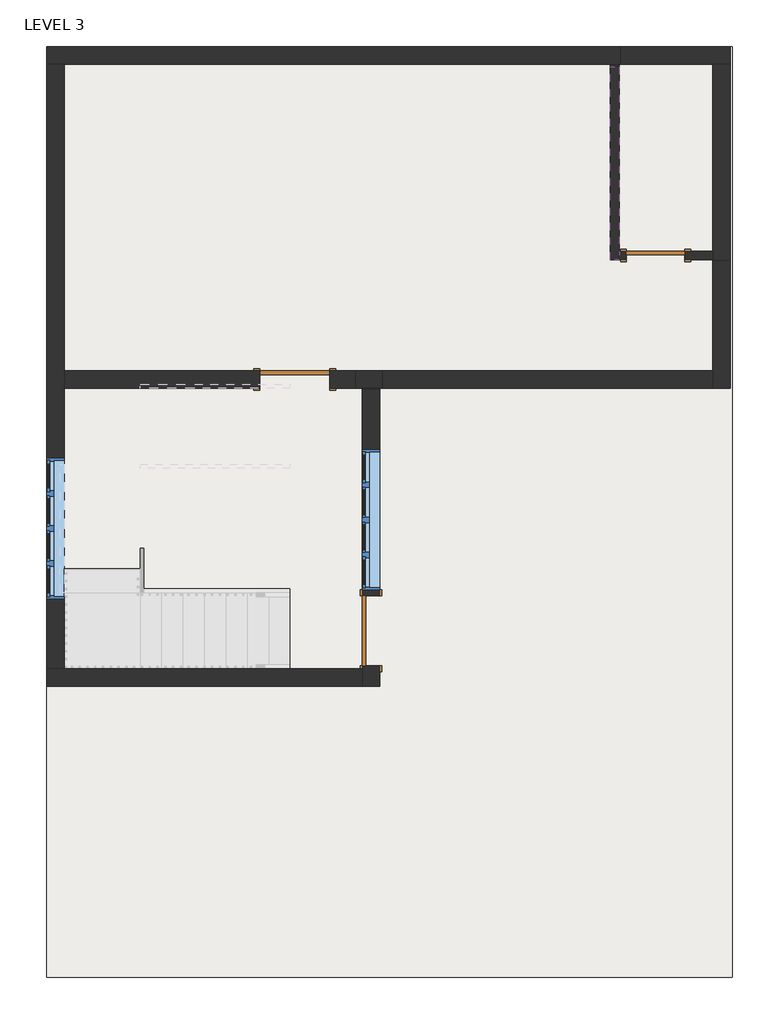
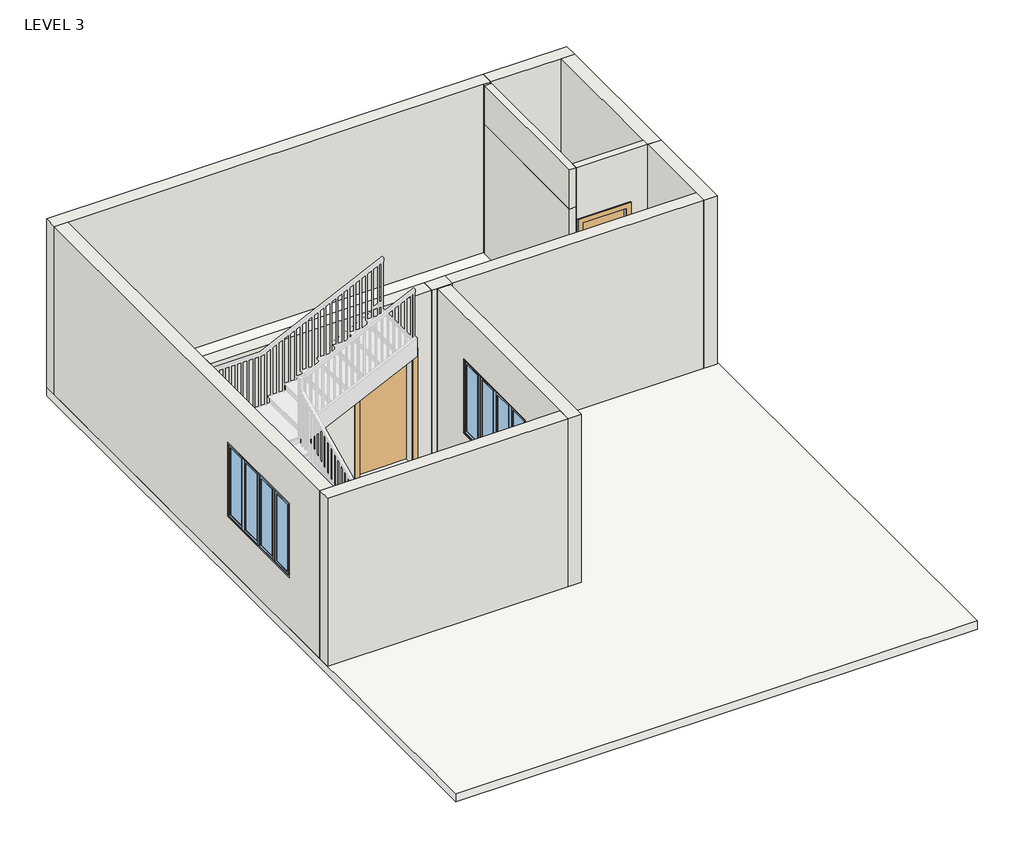
# One storey, part 1 of 3: 15 walls, 3 doors, 2 windows, 1 slab.
"""IFC4 building model written with IfcOpenShell, lengths in millimetres."""

from ifc_helpers import new_model, si_unit, frame, origin, place, context, project, spatial, polyline, outline, extrude, faceted_brep, transform, mapped, element, save
from components import door_feaa5179, door_f2b275c1, single_flush_door_3_89fc3733, window_5487fb6d

model = new_model("IFC4")

# Units and contexts
model_context = context("Model", 3, world=origin())
ifc_project = project(units=[si_unit("LENGTHUNIT", "METRE", prefix="MILLI")], contexts=[model_context])

# Site, building, storey
site = spatial("IfcSite", under=ifc_project)
building = spatial("IfcBuilding", under=site)
storey = spatial("IfcBuildingStorey", under=building, Name="LEVEL 3", Elevation=6248.4)

# Doors
placement = place(None, origin())
door_shape = door_feaa5179(model_context)
element("IfcDoor", 1, ObjectType="Door-Single-Flush_Panel_Double-Acting : 36\" x 80\"", at=placement, inside=storey, context=model_context, shape_type="MappedRepresentation", body=[
    mapped(door_shape, transform((-18715.7789184, -623.1399287, 6248.4), x_axis=(0.0, 1.0, 0.0), y_axis=(-1.0, 0.0, 0.0), z_axis=(0.0, 0.0, 1.0))),
])
door_2_shape = door_f2b275c1(model_context)
element("IfcDoor", 2, ObjectType="Single-Flush : door 2'6\"", at=placement, inside=storey, context=model_context, shape_type="MappedRepresentation", body=[
    mapped(door_2_shape, transform((-15001.0289184, 4272.7100713, 6248.4), x_axis=(-1.0, 0.0, 0.0), y_axis=(0.0, -1.0, 0.0), z_axis=(0.0, 0.0, 1.0))),
])
single_flush_door_3_shape = single_flush_door_3_89fc3733(model_context)
element("IfcDoor", 3, ObjectType="Single-Flush : door 3'", at=placement, inside=storey, context=model_context, shape_type="MappedRepresentation", body=[
    mapped(single_flush_door_3_shape, transform((-19706.3789184, 2653.4600713, 6248.4), x_axis=(1.0, 0.0, 0.0), y_axis=(0.0, 1.0, 0.0), z_axis=(0.0, 0.0, 1.0))),
])

# Slab
element("IfcSlab", 4, ObjectType="floor 6\"", at=placement, inside=storey, context=model_context, shape_type="SweptSolid", body=[
    extrude(outline(polyline([(-14004.0789184, 6996.8600713), (-14004.0789184, -5144.3399287), (-22944.8789184, -5144.3399287), (-22944.8789184, 6996.8600713), (-14004.0789184, 6996.8600713)])), frame((0.0, 0.0, 6096.0), z_axis=(0.0, 0.0, 1.0), x_axis=(1.0, 0.0, 0.0)), (0.0, 0.0, 1.0), 152.4),
])

# Walls
element("IfcWall", 5, ObjectType="WALL 4.5\"", at=placement, inside=storey, context=model_context, shape_type="Brep", body=[
    faceted_brep([(-15591.5789184, 6768.2600713, 6248.4), (-15591.5789184, 6730.1600713, 6248.4), (-15591.5789184, 6730.1600713, 8585.2), (-15591.5789184, 6730.1600713, 9296.4), (-15591.5789184, 6768.2600713, 9296.4), (-15477.2789184, 6768.2600713, 6248.4), (-15477.2789184, 6768.2600713, 9296.4), (-15477.2789184, 6730.1600713, 9296.4), (-15477.2789184, 6730.1600713, 8585.2), (-15477.2789184, 6730.1600713, 6248.4)], [[[0, 1, 2, 3, 4]], [[5, 6, 7, 8, 9]], [[1, 0, 5, 9]], [[4, 3, 7, 6]], [[0, 4, 6, 5]], [[1, 9, 8, 7, 3, 2]]]),
])
element("IfcWall", 6, ObjectType="WALL 4.5\"", at=placement, inside=storey, context=model_context, shape_type="Brep", body=[
    faceted_brep([(-14258.0789184, 4215.5600713, 9296.4), (-15477.2789184, 4215.5600713, 9296.4), (-15477.2789184, 4215.5600713, 8585.2), (-15477.2789184, 4215.5600713, 6248.4), (-15382.0289184, 4215.5600713, 6248.4), (-15382.0289184, 4215.5600713, 8280.4), (-14620.0289184, 4215.5600713, 8280.4), (-14620.0289184, 4215.5600713, 6248.4), (-14258.0789184, 4215.5600713, 6248.4), (-15477.2789184, 4329.8600713, 9296.4), (-14258.0789184, 4329.8600713, 9296.4), (-14258.0789184, 4329.8600713, 6248.4), (-14620.0289184, 4329.8600713, 6248.4), (-14620.0289184, 4329.8600713, 8280.4), (-15382.0289184, 4329.8600713, 8280.4), (-15382.0289184, 4329.8600713, 6248.4), (-15477.2789184, 4329.8600713, 6248.4)], [[[0, 1, 2, 3, 4, 5, 6, 7, 8]], [[9, 10, 11, 12, 13, 14, 15, 16]], [[3, 16, 15, 4]], [[11, 8, 7, 12]], [[1, 0, 10, 9]], [[0, 8, 11, 10]], [[14, 5, 4, 15]], [[6, 13, 12, 7]], [[13, 6, 5, 14]], [[1, 9, 16, 3, 2]]]),
])
element("IfcWall", 7, ObjectType="WALL 4.5\"", at=placement, inside=storey, context=model_context, shape_type="Brep", body=[
    faceted_brep([(-15591.5789184, 6730.1600713, 6248.4), (-15591.5789184, 4215.5600713, 6248.4), (-15591.5789184, 4215.5600713, 8585.2), (-15591.5789184, 6730.1600713, 8585.2), (-15477.2789184, 6730.1600713, 6248.4), (-15477.2789184, 6730.1600713, 8585.2), (-15477.2789184, 4215.5600713, 8585.2), (-15477.2789184, 4215.5600713, 6248.4), (-15477.2789184, 4329.8600713, 6248.4)], [[[0, 1, 2, 3]], [[4, 5, 6, 7, 8]], [[1, 0, 4, 8, 7]], [[3, 2, 6, 5]], [[0, 3, 5, 4]], [[2, 1, 7, 6]]]),
])
element("IfcWall", 8, ObjectType="WALL 4.5\"", at=placement, inside=storey, context=model_context, shape_type="Brep", body=[
    faceted_brep([(-15591.5789184, 6730.1600713, 8585.2), (-15591.5789184, 4215.5600713, 8585.2), (-15591.5789184, 4215.5600713, 9296.4), (-15591.5789184, 6730.1600713, 9296.4), (-15477.2789184, 6730.1600713, 8585.2), (-15477.2789184, 6730.1600713, 9296.4), (-15477.2789184, 4329.8600713, 9296.4), (-15477.2789184, 4215.5600713, 9296.4), (-15477.2789184, 4215.5600713, 8585.2)], [[[0, 1, 2, 3]], [[4, 5, 6, 7, 8]], [[1, 0, 4, 8]], [[3, 2, 7, 6, 5]], [[0, 3, 5, 4]], [[2, 1, 8, 7]]]),
])
element("IfcWall", 9, ObjectType="WALL 9\"", at=placement, inside=storey, context=model_context, shape_type="Brep", body=[
    faceted_brep([(-22944.8789184, 6768.2600713, 6248.4), (-22716.2789184, 6768.2600713, 6248.4), (-15591.5789184, 6768.2600713, 6248.4), (-15477.2789184, 6768.2600713, 6248.4), (-15464.5789184, 6768.2600713, 6248.4), (-15464.5789184, 6768.2600713, 9296.4), (-15477.2789184, 6768.2600713, 9296.4), (-15591.5789184, 6768.2600713, 9296.4), (-22716.2789184, 6768.2600713, 9296.4), (-22944.8789184, 6768.2600713, 9296.4), (-22944.8789184, 6996.8600713, 6248.4), (-22944.8789184, 6996.8600713, 9296.4), (-15464.5789184, 6996.8600713, 9296.4), (-15464.5789184, 6996.8600713, 6248.4)], [[[0, 1, 2, 3, 4, 5, 6, 7, 8, 9]], [[10, 11, 12, 13]], [[4, 3, 2, 1, 0, 10, 13]], [[5, 4, 13, 12]], [[0, 9, 11, 10]], [[9, 8, 7, 6, 5, 12, 11]]]),
])
element("IfcWall", 10, ObjectType="WALL 9\"", at=placement, inside=storey, context=model_context, shape_type="Brep", body=[
    faceted_brep([(-14258.0789184, 6768.2600713, 6248.4), (-14258.0789184, 4329.8600713, 6248.4), (-14258.0789184, 4215.5600713, 6248.4), (-14258.0789184, 4202.8600713, 6248.4), (-14258.0789184, 4202.8600713, 9296.4), (-14258.0789184, 4215.5600713, 9296.4), (-14258.0789184, 4329.8600713, 9296.4), (-14258.0789184, 6768.2600713, 9296.4), (-14029.4789184, 6768.2600713, 6248.4), (-14029.4789184, 6768.2600713, 9296.4), (-14029.4789184, 4202.8600713, 9296.4), (-14029.4789184, 4202.8600713, 6248.4)], [[[0, 1, 2, 3, 4, 5, 6, 7]], [[8, 9, 10, 11]], [[3, 2, 1, 0, 8, 11]], [[4, 3, 11, 10]], [[0, 7, 9, 8]], [[7, 6, 5, 4, 10, 9]]]),
])
element("IfcWall", 11, ObjectType="WALL 9\"", at=placement, inside=storey, context=model_context, shape_type="SweptSolid", body=[
    extrude(outline(polyline([(-18563.3789184, 2767.7600713), (-14258.0789184, 2767.7600713), (-14258.0789184, 2539.1600713), (-18563.3789184, 2539.1600713), (-18563.3789184, 2767.7600713)])), frame((0.0, 0.0, 6248.4), z_axis=(0.0, 0.0, 1.0), x_axis=(1.0, 0.0, 0.0)), (0.0, 0.0, 1.0), 3048.0),
])
element("IfcWall", 12, ObjectType="WALL 9\"", at=placement, inside=storey, context=model_context, shape_type="SweptSolid", body=[
    extrude(outline(polyline([(-18830.0789184, 2526.4600713), (-18830.0789184, 2539.1600713), (-18601.4789184, 2539.1600713), (-18601.4789184, 2526.4600713), (-18830.0789184, 2526.4600713)])), frame((0.0, 0.0, 6248.4), z_axis=(0.0, 0.0, 1.0), x_axis=(1.0, 0.0, 0.0)), (0.0, 0.0, 1.0), 3048.0),
])
element("IfcWall", 13, ObjectType="WALL 9\"", at=placement, inside=storey, context=model_context, shape_type="Brep", body=[
    faceted_brep([(-18830.0789184, -1118.4399287, 6248.4), (-22716.2789184, -1118.4399287, 6248.4), (-22944.8789184, -1118.4399287, 6248.4), (-22944.8789184, -1118.4399287, 9296.4), (-22716.2789184, -1118.4399287, 9296.4), (-19769.8789184, -1118.4399287, 9296.4), (-18830.0789184, -1118.4399287, 9296.4), (-18830.0789184, -1347.0399287, 6248.4), (-18830.0789184, -1347.0399287, 9296.4), (-22944.8789184, -1347.0399287, 9296.4), (-22944.8789184, -1347.0399287, 6248.4)], [[[0, 1, 2, 3, 4, 5, 6]], [[7, 8, 9, 10]], [[2, 1, 0, 7, 10]], [[0, 6, 8, 7]], [[3, 2, 10, 9]], [[6, 5, 4, 3, 9, 8]]]),
])
element("IfcWall", 14, ObjectType="WALL 9\"", at=placement, inside=storey, context=model_context, shape_type="Brep", body=[
    faceted_brep([(-22716.2789184, -1118.4399287, 6248.4), (-22716.2789184, 2539.1600713, 6248.4), (-22716.2789184, 2767.7600713, 6248.4), (-22716.2789184, 6768.2600713, 6248.4), (-22716.2789184, 6768.2600713, 9296.4), (-22716.2789184, 2767.7600713, 9296.4), (-22716.2789184, 2539.1600713, 9296.4), (-22716.2789184, -1118.4399287, 9296.4), (-22716.2789184, 1624.7600713, 8509.0), (-22716.2789184, 1624.7600713, 7162.8), (-22716.2789184, -204.0399287, 7162.8), (-22716.2789184, -204.0399287, 8509.0), (-22944.8789184, -1118.4399287, 6248.4), (-22944.8789184, -1118.4399287, 9296.4), (-22944.8789184, 6768.2600713, 9296.4), (-22944.8789184, 6768.2600713, 6248.4), (-22944.8789184, 1624.7600713, 8509.0), (-22944.8789184, -204.0399287, 8509.0), (-22944.8789184, -204.0399287, 7162.8), (-22944.8789184, 1624.7600713, 7162.8)], [[[0, 1, 2, 3, 4, 5, 6, 7], [8, 9, 10, 11]], [[12, 13, 14, 15], [16, 17, 18, 19]], [[3, 2, 1, 0, 12, 15]], [[0, 7, 13, 12]], [[4, 3, 15, 14]], [[7, 6, 5, 4, 14, 13]], [[9, 8, 16, 19]], [[10, 9, 19, 18]], [[11, 10, 18, 17]], [[8, 11, 17, 16]]]),
])
element("IfcWall", 15, ObjectType="WALL 9\"", at=placement, inside=storey, context=model_context, shape_type="Brep", body=[
    faceted_brep([(-18830.0789184, 2526.4600713, 6248.4), (-18830.0789184, -165.9399287, 6248.4), (-18830.0789184, -165.9399287, 8280.4), (-18830.0789184, -1080.3399287, 8280.4), (-18830.0789184, -1080.3399287, 6248.4), (-18830.0789184, -1118.4399287, 6248.4), (-18830.0789184, -1347.0399287, 6248.4), (-18830.0789184, -1347.0399287, 9296.4), (-18830.0789184, -1118.4399287, 9296.4), (-18830.0789184, 2526.4600713, 9296.4), (-18830.0789184, 1739.0600713, 8509.0), (-18830.0789184, -89.7399287, 8509.0), (-18830.0789184, -89.7399287, 7162.8), (-18830.0789184, 1739.0600713, 7162.8), (-18601.4789184, -165.9399287, 8280.4), (-18601.4789184, -165.9399287, 6248.4), (-18601.4789184, 2526.4600713, 6248.4), (-18601.4789184, 2526.4600713, 9296.4), (-18601.4789184, -1347.0399287, 9296.4), (-18601.4789184, -1347.0399287, 6248.4), (-18601.4789184, -1080.3399287, 6248.4), (-18601.4789184, -1080.3399287, 8280.4), (-18601.4789184, 1739.0600713, 8509.0), (-18601.4789184, 1739.0600713, 7162.8), (-18601.4789184, -89.7399287, 7162.8), (-18601.4789184, -89.7399287, 8509.0)], [[[0, 1, 2, 3, 4, 5, 6, 7, 8, 9], [10, 11, 12, 13]], [[14, 15, 16, 17, 18, 19, 20, 21], [22, 23, 24, 25]], [[20, 19, 6, 5, 4]], [[16, 15, 1, 0]], [[0, 9, 17, 16]], [[7, 6, 19, 18]], [[9, 8, 7, 18, 17]], [[22, 25, 11, 10]], [[25, 24, 12, 11]], [[24, 23, 13, 12]], [[23, 22, 10, 13]], [[2, 1, 15, 14]], [[3, 2, 14, 21]], [[4, 3, 21, 20]]]),
])
element("IfcWall", 16, ObjectType="WALL 9\"", at=placement, inside=storey, context=model_context, shape_type="Brep", body=[
    faceted_brep([(-18563.3789184, 2767.7600713, 6248.4), (-18918.9789184, 2767.7600713, 6248.4), (-18918.9789184, 2767.7600713, 9296.4), (-18563.3789184, 2767.7600713, 9296.4), (-18563.3789184, 2539.1600713, 6248.4), (-18563.3789184, 2539.1600713, 9296.4), (-18601.4789184, 2539.1600713, 9296.4), (-18830.0789184, 2539.1600713, 9296.4), (-18918.9789184, 2539.1600713, 9296.4), (-18918.9789184, 2539.1600713, 6248.4), (-18830.0789184, 2539.1600713, 6248.4), (-18601.4789184, 2539.1600713, 6248.4)], [[[0, 1, 2, 3]], [[4, 5, 6, 7, 8, 9, 10, 11]], [[1, 0, 4, 11, 10, 9]], [[2, 1, 9, 8]], [[0, 3, 5, 4]], [[3, 2, 8, 7, 6, 5]]]),
])
element("IfcWall", 17, ObjectType="WALL 9\"", at=placement, inside=storey, context=model_context, shape_type="Brep", body=[
    faceted_brep([(-15464.5789184, 6768.2600713, 6248.4), (-14258.0789184, 6768.2600713, 6248.4), (-14029.4789184, 6768.2600713, 6248.4), (-14029.4789184, 6768.2600713, 9296.4), (-14258.0789184, 6768.2600713, 9296.4), (-15464.5789184, 6768.2600713, 9296.4), (-15464.5789184, 6996.8600713, 6248.4), (-15464.5789184, 6996.8600713, 9296.4), (-14029.4789184, 6996.8600713, 9296.4), (-14029.4789184, 6996.8600713, 6248.4)], [[[0, 1, 2, 3, 4, 5]], [[6, 7, 8, 9]], [[2, 1, 0, 6, 9]], [[0, 5, 7, 6]], [[3, 2, 9, 8]], [[5, 4, 3, 8, 7]]]),
])
element("IfcWall", 18, ObjectType="WALL 9\"", at=placement, inside=storey, context=model_context, shape_type="Brep", body=[
    faceted_brep([(-14258.0789184, 4202.8600713, 6248.4), (-14258.0789184, 2767.7600713, 6248.4), (-14258.0789184, 2539.1600713, 6248.4), (-14258.0789184, 2539.1600713, 9296.4), (-14258.0789184, 2767.7600713, 9296.4), (-14258.0789184, 4202.8600713, 9296.4), (-14029.4789184, 4202.8600713, 6248.4), (-14029.4789184, 4202.8600713, 9296.4), (-14029.4789184, 2539.1600713, 9296.4), (-14029.4789184, 2539.1600713, 6248.4)], [[[0, 1, 2, 3, 4, 5]], [[6, 7, 8, 9]], [[2, 1, 0, 6, 9]], [[0, 5, 7, 6]], [[3, 2, 9, 8]], [[5, 4, 3, 8, 7]]]),
])
element("IfcWall", 19, ObjectType="WALL 9\"", at=placement, inside=storey, context=model_context, shape_type="Brep", body=[
    faceted_brep([(-18918.9789184, 2767.7600713, 6248.4), (-19249.1789184, 2767.7600713, 6248.4), (-19249.1789184, 2767.7600713, 8280.4), (-20163.5789184, 2767.7600713, 8280.4), (-20163.5789184, 2767.7600713, 6248.4), (-22716.2789184, 2767.7600713, 6248.4), (-22716.2789184, 2767.7600713, 9296.4), (-18918.9789184, 2767.7600713, 9296.4), (-19249.1789184, 2539.1600713, 8280.4), (-19249.1789184, 2539.1600713, 6248.4), (-18918.9789184, 2539.1600713, 6248.4), (-18918.9789184, 2539.1600713, 9296.4), (-19769.8789184, 2539.1600713, 9296.4), (-22716.2789184, 2539.1600713, 9296.4), (-22716.2789184, 2539.1600713, 6248.4), (-20163.5789184, 2539.1600713, 6248.4), (-20163.5789184, 2539.1600713, 8280.4)], [[[0, 1, 2, 3, 4, 5, 6, 7]], [[8, 9, 10, 11, 12, 13, 14, 15, 16]], [[15, 14, 5, 4]], [[10, 9, 1, 0]], [[0, 7, 11, 10]], [[6, 5, 14, 13]], [[7, 6, 13, 12, 11]], [[4, 3, 16, 15]], [[3, 2, 8, 16]], [[2, 1, 9, 8]]]),
])

# Windows
window_shape = window_5487fb6d(model_context)
element("IfcWindow", 20, ObjectType="Window-Casement-Multi-Sash-Horizontal : 72\" x 53\"", at=placement, inside=storey, context=model_context, shape_type="MappedRepresentation", body=[
    mapped(window_shape, transform((-18715.7789184, 824.6600713, 6248.4), x_axis=(0.0, 1.0, 0.0), y_axis=(-1.0, 0.0, 0.0), z_axis=(0.0, 0.0, 1.0))),
])
element("IfcWindow", 21, ObjectType="Window-Casement-Multi-Sash-Horizontal : 72\" x 53\"", at=placement, inside=storey, context=model_context, shape_type="MappedRepresentation", body=[
    mapped(window_shape, transform((-22830.5789184, 710.3600713, 6248.4), x_axis=(0.0, 1.0, 0.0), y_axis=(-1.0, 0.0, 0.0), z_axis=(0.0, 0.0, 1.0))),
])

save(model, "model.ifc")

# Revit data of these elements
# Type "Door-Single-Flush_Panel_Double-Acting : 36\" x 80\""
#   Type Mark = "11"
#   Construction Type Id = "DOOR"
#   Assembly Code = "C1020300"
#   Analytic Construction = "Wooden"
#   Thickness = 0' - 2"
#   Thermal Resistance (R) = 2.5876 (h·ft²·°F)/BTU
#   Swing Angle [instance default] = 90.00°
#   Heat Transfer Coefficient (U) = 0.3865 BTU/(h·ft²·°F)
#   Height = 6' - 8"
#   Trim Projection Ext. = 0' - 1"
#   Trim Projection Int. = 0' - 1"
#   Trim Width Ext. = 0' - 3"
#   Trim Width Int. = 0' - 3"
#   Width = 3' - 0"
#   Define Thermal Properties by = 1
#   Trim Material = Paint - Sienna
#   Panel Material = Wood - Birch - Solid Stained Light Low Gloss
#   Visual Light Transmittance = 0
#   Solar Heat Gain Coefficient = 0
#   Function = (empty or 0)
#   Wall Closure = (empty or 0)
# Type "Single-Flush : door 2'6\""
#   Type Mark = "10"
#   Construction Type Id = "MDOOR"
#   Assembly Code = "C1020"
#   Analytic Construction = "Metal"
#   Thickness = 0' - 2"
#   Heat Transfer Coefficient (U) = 0.651978 BTU/(h·ft²·°F)
#   Height = 6' - 8"
#   Trim Projection Ext = 0' - 1"
#   Trim Projection Int = 0' - 1"
#   Trim Width = 0' - 3"
#   Width = 2' - 6"
#   Define Thermal Properties by = 1
#   Door Material = Door - Panel
#   Frame Material = Door - Frame
#   Visual Light Transmittance = 0
#   Solar Heat Gain Coefficient = 0
#   Function = (empty or 0)
#   Wall Closure = (empty or 0)
# Type "Single-Flush : door 3'"
#   Type Mark = "9"
#   Construction Type Id = "MDOOR"
#   Assembly Code = "C1020"
#   Analytic Construction = "Metal"
#   Thickness = 0' - 2"
#   Heat Transfer Coefficient (U) = 0.651978 BTU/(h·ft²·°F)
#   Height = 6' - 8"
#   Trim Projection Ext = 0' - 1"
#   Trim Projection Int = 0' - 1"
#   Trim Width = 0' - 3"
#   Width = 3' - 0"
#   Define Thermal Properties by = 1
#   Door Material = Door - Panel
#   Frame Material = Door - Frame
#   Visual Light Transmittance = 0
#   Solar Heat Gain Coefficient = 0
#   Function = (empty or 0)
#   Wall Closure = (empty or 0)
# Type "floor 6\""
#   Assembly Code = "B1010"
#   Function = 0
#   Layers, outside or top first: 0' - 6" no material (function 1)
# Type "WALL 4.5\""
#   Assembly Code = "B2010"
#   Layers, outside or top first: 0' - 4 1/2" no material (function 1)
# Type "WALL 9\""
#   Assembly Code = "B2010"
#   Layers, outside or top first: 0' - 9" no material (function 1)
# Type "Window-Casement-Multi-Sash-Horizontal : 72\" x 53\""
#   Type Mark = "18"
#   Fire Rating = "0.5h"
#   Assembly Code = "B2020100"
#   Analytic Construction = "Double glazing - domestic"
#   Window Inset [instance default] = 0' - 0 5/8"
#   Wall Thickness [instance default] = 0' - 6"
#   Visual Light Transmittance = 0.81
#   Thermal Resistance (R) = 1.8146 (h·ft²·°F)/BTU
#   Solar Heat Gain Coefficient = 0.76
#   Rough Width = 6' - 0 1/2"
#   Rough Height = 4' - 5 1/2"
#   Open Window Width = 1' - 6"
#   Heat Transfer Coefficient (U) = 0.5511 BTU/(h·ft²·°F)
#   Height = 4' - 5"
#   Frame Gap 3 [instance default] = 0' - 1 83/128"
#   Frame Gap 2 [instance default] = 0' - 0 5/8"
#   Frame Gap 1 = 0' - 1 51/128"
#   Default Sill Height = 3' - 0"
#   Width = 6' - 0"
#   Frame Material = Metal - Aluminum
#   Glass Panel Material = Glass
#   Wall Closure = (empty or 0)
# Element 1 (IfcDoor, "Door-Single-Flush_Panel_Double-Acting : 36\" x 80\"")
#   Swing Angle = 90.00°
#   Phase Created = New Construction
#   Materials on its faces: "Paint - Sienna", "Wood - Birch - Solid Stained Light Low Gloss"
# Element 2 (IfcDoor, "Single-Flush : door 2'6\"")
#   Phase Created = New Construction
#   Materials on its faces: "Door - Frame", "Door - Panel"
# Element 3 (IfcDoor, "Single-Flush : door 3'")
#   Phase Created = New Construction
#   Materials on its faces: "Door - Frame", "Door - Panel"
# Element 4 (IfcSlab, "floor 6\"")
#   Height Offset From Level = 0' - 0"
#   Phase Created = New Construction
#   Materials on its faces: "light shade", "Default Floor", "MULTI F"
# Elements 5, 6 (IfcWall, "WALL 4.5\"")
#   Top Offset = 0' - 0"
#   Base Offset = 0' - 0"
#   Unconnected Height = 10' - 0"
#   wall height = 10' - 0"
#   Phase Created = New Construction
#   Base Constraint = LEVEL 3
#   Materials on its faces: "Default Wall", "1 wall", "diff"
# Element 7 (IfcWall, "WALL 4.5\"")
#   Top Offset = 0' - 0"
#   Base Offset = 0' - 0"
#   Unconnected Height = 7' - 8"
#   wall height = 7' - 8"
#   Phase Created = New Construction
#   Base Constraint = LEVEL 3
#   Materials on its faces: "Default Wall", "1 wall", "diff"
# Element 8 (IfcWall, "WALL 4.5\"")
#   built-in parameter 1001111 = 7' - 8"
#   Top Offset = 0' - 0"
#   Base Offset = 7' - 8"
#   Unconnected Height = 2' - 4"
#   wall height = 2' - 4"
#   Phase Created = New Construction
#   Base Constraint = LEVEL 3
#   Materials on its faces: "Default Wall", "1 wall", "diff"
# Elements 9, 13, 15, 18 (IfcWall, "WALL 9\"")
#   Top Offset = 0' - 0"
#   Base Offset = 0' - 0"
#   Unconnected Height = 10' - 0"
#   wall height = 10' - 0"
#   Phase Created = New Construction
#   Base Constraint = LEVEL 3
#   Materials on its faces: "Default Wall", "7f 678e", "1 wall"
# Element 10 (IfcWall, "WALL 9\"")
#   Top Offset = 0' - 0"
#   Base Offset = 0' - 0"
#   Unconnected Height = 10' - 0"
#   wall height = 10' - 0"
#   Phase Created = New Construction
#   Base Constraint = LEVEL 3
#   Materials on its faces: "Default Wall", "diff", "7f 678e"
# Elements 11, 14 (IfcWall, "WALL 9\"")
#   Top Offset = 0' - 0"
#   Base Offset = 0' - 0"
#   Unconnected Height = 10' - 0"
#   wall height = 10' - 0"
#   Phase Created = New Construction
#   Base Constraint = LEVEL 3
#   Materials on its faces: "Default Wall", "1 wall", "7f 678e"
# Elements 12, 16, 19 (IfcWall, "WALL 9\"")
#   Top Offset = 0' - 0"
#   Base Offset = 0' - 0"
#   Unconnected Height = 10' - 0"
#   wall height = 10' - 0"
#   Phase Created = New Construction
#   Base Constraint = LEVEL 3
#   Materials on its faces: "Default Wall", "1 wall"
# Element 17 (IfcWall, "WALL 9\"")
#   Top Offset = 0' - 0"
#   Base Offset = 0' - 0"
#   Unconnected Height = 10' - 0"
#   wall height = 10' - 0"
#   Phase Created = New Construction
#   Base Constraint = LEVEL 3
#   Materials on its faces: "Default Wall", "7f 678e", "diff"
# Element 20 (IfcWindow, "Window-Casement-Multi-Sash-Horizontal : 72\" x 53\"")
#   Mark = "22"
#   Window Inset = 0' - 0 5/8"
#   Frame Gap 3 = 0' - 1 83/128"
#   Frame Gap 2 = 0' - 0 5/8"
#   Phase Created = New Construction
#   Materials on its faces: "Metal - Aluminum", "Glass"
# Element 21 (IfcWindow, "Window-Casement-Multi-Sash-Horizontal : 72\" x 53\"")
#   Mark = "23"
#   Window Inset = 0' - 0 5/8"
#   Frame Gap 3 = 0' - 1 83/128"
#   Frame Gap 2 = 0' - 0 5/8"
#   Phase Created = New Construction
#   Materials on its faces: "Metal - Aluminum", "Glass"
# Materials
#   "Paint - Sienna": colour RGB 118 70 51, transparency 0, Cost = 0
#   "Wood - Birch - Solid Stained Light Low Gloss": class "Wood", colour RGB 210 159 95, transparency 0, Cost = 0
#   "Door - Panel": class "Wood", colour RGB 210 159 95, transparency 0, Cost = 0
#   "Door - Frame": colour RGB 118 70 51, transparency 0, Cost = 0
#   "Metal - Aluminum": class "Metal", colour RGB 247 247 247, transparency 0
#   "Glass": class "Glass", colour RGB 0 128 192, transparency 0.75, Description = "Soda Lime Glass", Cost = 0
#   "light shade": class "Generic", colour RGB 120 120 120, transparency 0, Cost = 0
#   "Default Floor": colour RGB 128 128 128, transparency 0, Cost = 0
#   "MULTI F": class "Generic", colour RGB 120 120 120, transparency 0, Cost = 0
#   "Default Wall": colour RGB 128 128 128, transparency 0, Cost = 0
#   "1 wall": class "Glass", colour RGB 0 0 255, transparency 0.75, Cost = 0
#   "diff": class "Generic", colour RGB 120 120 120, transparency 0, Cost = 0
#   "7f 678e": class "Generic", colour RGB 120 120 120, transparency 0, Cost = 0
